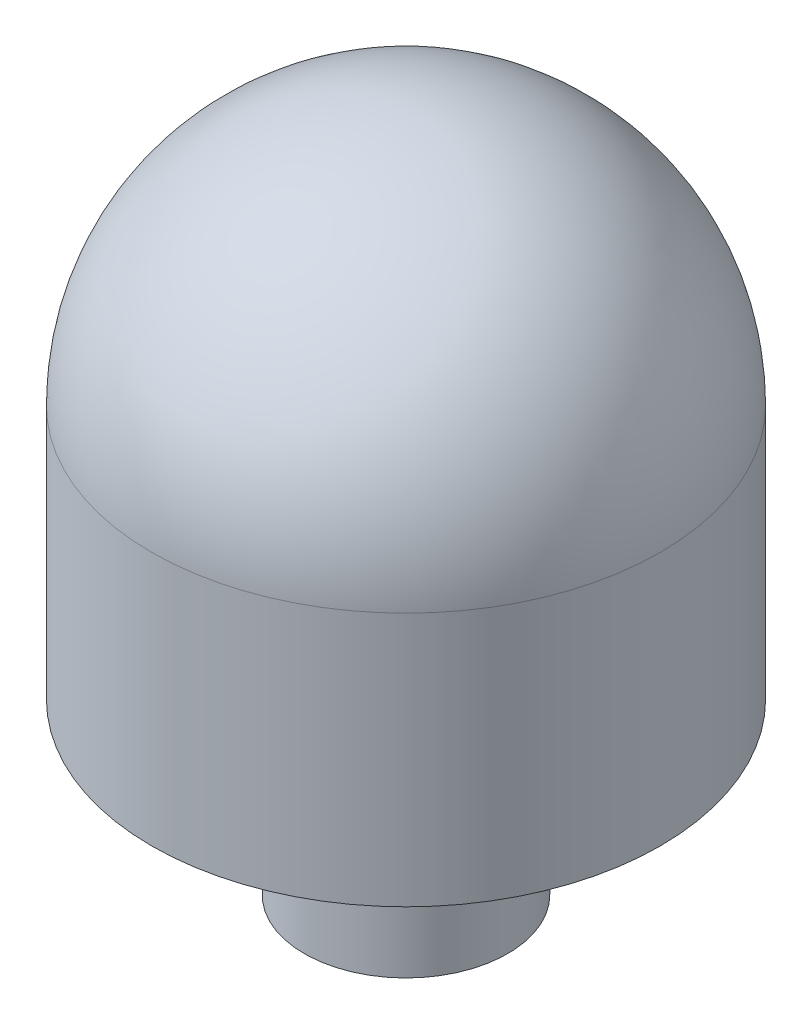
SolidWorks part; units mm, degrees
material "Plain Carbon Steel"
ref_plane "Front Plane" through (0, 0, 0) normal (0, 0, 1) x (1, 0, 0)
ref_plane "Top Plane" through (0, 0, 0) normal (0, 1, 0) x (1, 0, 0)
ref_plane "Right Plane" through (0, 0, 0) normal (1, 0, 0) x (0, 0, -1)
sketch "Pin Profile Sketch" plane through (0, 0, 0) normal (0, 0, 1) x (1, 0, 0)
  line L0 (0, 0) -> (6, 0)
  line L1 (6, 0) -> (6, 10)
  line L2 (6, 10) -> (15, 10)
  line L3 (15, 10) -> (15, 25)
  line L4 (0, 40) -> (0, 0)
  arc A0 (15, 25) -> (0, 40) centre (0, 25) ccw
  dimension "D3" = 10
  dimension "D1" = 6
  dimension "D2" = 15
  dimension "D4" = 25
revolve "Pin Body Revolve" add sketch "Pin Profile Sketch" angle 360 about L4
